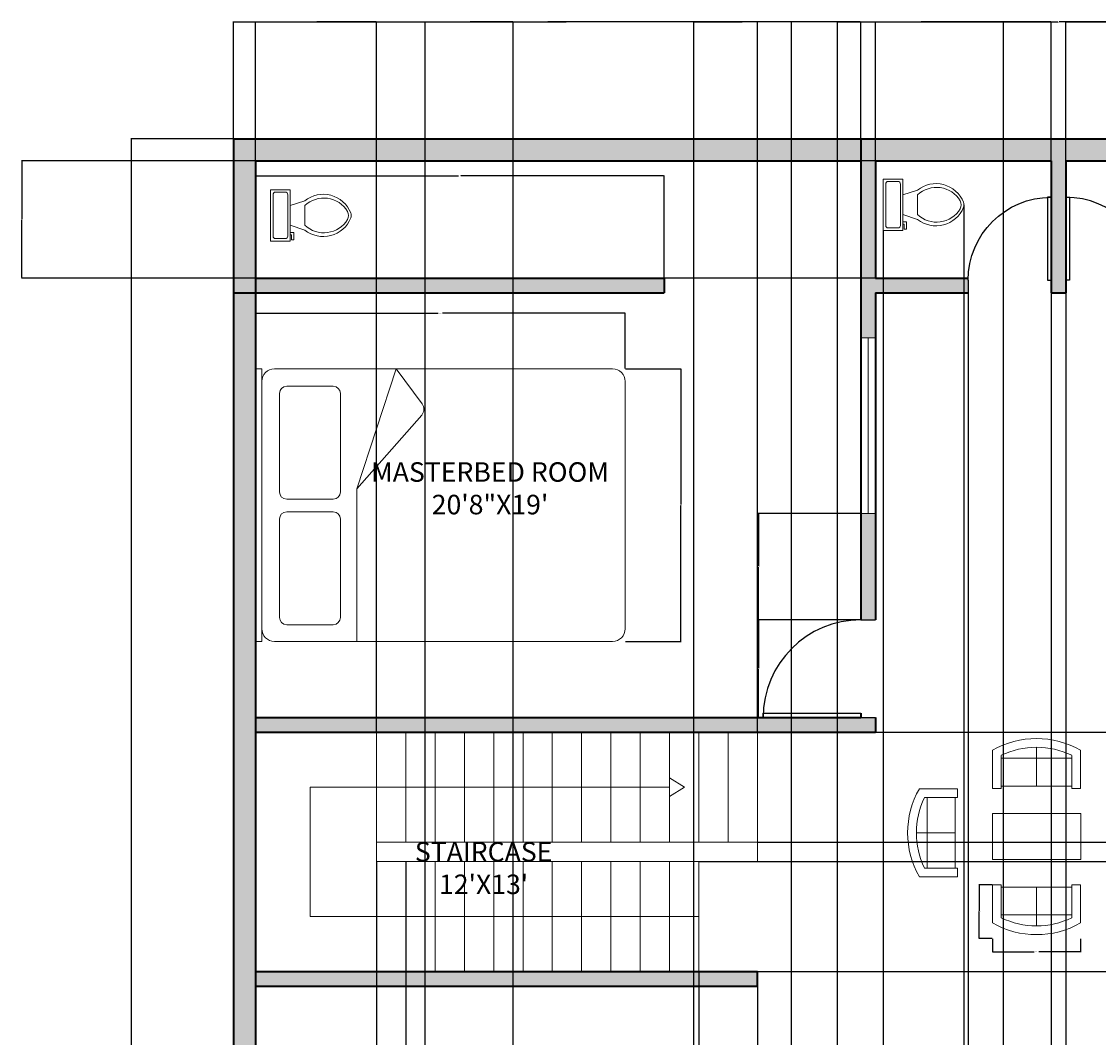
# Model space of a CAD drawing. Units: inches. Extents: x -89 to 661, y -827 to 77.
# Tile 4 of 5: x -89 to 353, y -339 to 77. Entities that reach past the tile are written whole.
import ezdxf

# ---------------------------------------------------------------- set-up
doc = ezdxf.new("R2010")
doc.units = ezdxf.units.IN
doc.header["$MEASUREMENT"] = 0
for name, color, linetype, lineweight in [('A-ANNO-DIMS', 2, 'Continuous', 18), ('A-AREA-IDEN', 7, 'Continuous', 18), ('A-FLOR-FIXT', 9, 'Continuous', 18), ('A-FLOR-STRS', 6, 'Continuous', 18), ('A-FURN', 34, 'Continuous', 18), ('A-GLAZ', 5, 'Continuous', 18), ('A-WALL', 7, 'Continuous', 35), ('A-WALL-PATT', 30, 'Continuous', 13), ('DOOR', 5, 'Continuous', 25)]:
    doc.layers.add(name, color=color, linetype=linetype, lineweight=lineweight)
doc.styles.get("Standard").update_dxf_attribs({"font": 'arial.ttf'})
doc.dimstyles.get("Standard").update_dxf_attribs({"dimtxt": 0.18, "dimasz": 0.18, "dimexe": 0.18, "dimexo": 0.0625, "dimgap": 0.09, "dimtad": 0, "dimtih": 1, "dimtoh": 1, "dimdec": 4, "dimzin": 0, "dimdsep": 46, "dimtxsty": 'Standard', "dimcen": 0.09, "dimadec": 0, "dimazin": 0, "dimtfac": 1, "dimtdec": 4, "dimtofl": 0, "dimtmove": 0, "dimatfit": 3, "dimfxl": 1, "dimtolj": 1, "dimtzin": 0, "dimarcsym": 0})

# ---------------------------------------------------------------- blocks, each defined once
blk = doc.blocks.new('*U7')
for p, q in [((0, 0), (0, -6)), ((40, 0), (40, -6))]:
    blk.add_line(p, q)
blk.add_lwpolyline([(0, 0), (0, 40), (1.75, 40), (1.75, 0)], close=True)
blk.add_arc((0, 0), 40, 0, 90)
blk = doc.blocks.new('A$C164346CA')
for p, q in [((0, 2.035), (0, 2)), ((1.5, 2.035), (0, 2.035)), ((1.5, 2), (1.5, 2.035)), ((1.5, 2), (0, 2)), ((0, 1.93), (0, 0.07)), ((0.6731, 1.9024), (0.1319, 1.9024)), ((1.364, 1.9024), (0.8228, 1.9024)), ((1.5, 0.07), (1.5, 1.93)), ((0.0919, 1.8624), (0.0919, 1.6069)), ((0.7131, 1.6069), (0.7131, 1.8624)), ((0.7828, 1.8624), (0.7828, 1.6069)), ((1.404, 1.6069), (1.404, 1.8624)), ((0.1319, 1.5669), (0.6731, 1.5669)), ((0.8228, 1.5669), (1.364, 1.5669)), ((0.8395, 1.4761), (0, 1.4761)), ((0.8395, 1.4761), (1.2448, 1.12)), ((1.5, 1.2611), (0.8395, 1.4761)), ((1.3077, 1.1175), (1.5, 1.2611)), ((0.07, 0), (1.43, 0))]:
    blk.add_line(p, q)
for centre, radius, start, end in [((0.07, 1.93), 0.07, 90, 180), ((1.43, 1.93), 0.07, 0, 90), ((0.1319, 1.8624), 0.04, 90, 180), ((0.6731, 1.8624), 0.04, 0, 90), ((0.8228, 1.8624), 0.04, 90, 180), ((1.364, 1.8624), 0.04, 0, 90), ((0.1319, 1.6069), 0.04, 180, 270), ((0.6731, 1.6069), 0.04, 270, 0), ((0.8228, 1.6069), 0.04, 180, 270), ((1.364, 1.6069), 0.04, 270, 0), ((1.2778, 1.1575), 0.05, 228.69584, 306.75789), ((0.07, 0.07), 0.07, 180, 270), ((1.43, 0.07), 0.07, 270, 0)]:
    blk.add_arc(centre, radius, start, end)
blk = doc.blocks.new('A$C01575E38')
for p, q in [((0, 0), (0, 0.65)), ((0, 0), (0, 0.65)), ((0.15, 0), (0.15, 0.563)), ((0.15, 0), (0.15, 0.563)), ((0.75, 0.039), (0.75, 0.7)), ((0.75, 0.039), (0.75, 0.7)), ((1.35, 0), (1.35, 0.563)), ((1.35, 0), (1.35, 0.563)), ((1.5, 0.65), (1.5, 0)), ((1.5, 0.65), (1.5, 0)), ((0.15, 0.515), (1.35, 0.515)), ((0.15, 0.515), (1.35, 0.515)), ((0.15, 0), (0, 0)), ((0.15, 0), (0, 0)), ((0.15, 0.039), (1.35, 0.039)), ((0.15, 0.039), (1.35, 0.039)), ((1.5, 0), (1.35, 0)), ((1.5, 0), (1.35, 0))]:
    blk.add_line(p, q)
for centre, radius, start, end in [((0.75, -0.656), 1.506, 60.1372, 119.8628), ((0.75, -0.656), 1.506, 60.1372, 119.8628), ((0.75, -0.685), 1.385, 64.3208, 115.6792), ((0.75, -0.685), 1.385, 64.3208, 115.6792)]:
    blk.add_arc(centre, radius, start, end)
blk = doc.blocks.new('*U15')
for p, q in [((9.5, -6), (9.5, -2)), ((-10, -8.5), (-8, -8.5)), ((-10, -9.5), (-10, -8.5)), ((-8, -8.5), (-8, -8)), ((-7, -8), (-7, -9.5)), ((-4, -8), (-6, -14)), ((4, -8), (6, -14)), ((-7, -9.5), (-10, -9.5)), ((4, -14), (-4, -14))]:
    blk.add_line(p, q)
blk.add_lwpolyline([(10.5, -8), (10.5, 0), (-10.5, 0), (-10.5, -8)], close=True)
for points in [[(-9.5, -2), (-9.5, -6)], [(8.5, -1), (-8.5, -1)], [(-8.5, -7), (8.5, -7)]]:
    blk.add_lwpolyline(points)
for centre, radius, start, end in [((-8.62, -1.88), 0.884, 81.8699, 188.1301), ((8.62, -1.88), 0.884, 351.8699, 98.1301), ((-8.62, -6.12), 0.884, 171.8699, 278.1301), ((8.62, -6.12), 0.884, 261.8699, 8.1301), ((3.52, -21.58), 12.17, 141.4691, 247.9714), ((4.2, -21.82), 11.33, 136.3677, 238.9468), ((-3.52, -21.58), 12.17, 292.0284, 38.5307), ((-4.2, -21.82), 11.33, 301.053, 43.6321), ((0, -27.88), 4, 245.7318, 294.2682), ((0, -29), 4, 254.8605, 285.1395)]:
    blk.add_arc(centre, radius, start, end)
blk = doc.blocks.new('WIN-72-NOM')
for p, q in [((0, 6), (0, 0)), ((0, 6), (71.86, 6)), ((71.86, 6), (71.86, 0)), ((0, 3), (71.86, 3)), ((0, 0), (71.86, 0))]:
    blk.add_line(p, q)
blk = doc.blocks.new('*D17')
at = {"layer": 'A-ANNO-DIMS', "color": 0, "lineweight": -2, "transparency": 16777216}
for p, q in [((309.15, -298.56), (309.15, -304.09)), ((345.23, -298.56), (345.23, -304.09)), ((309.33, -303.91), (326.24, -303.91)), ((345.05, -303.91), (328.14, -303.91))]:
    blk.add_line(p, q, dxfattribs=at)
at = {"layer": 'A-ANNO-DIMS', "color": 0, "transparency": 16777216}
for points in [[(309.33, -303.88), (309.33, -303.94), (309.15, -303.91)], [(345.05, -303.88), (345.05, -303.94), (345.23, -303.91)]]:
    blk.add_solid(points, dxfattribs=at)
at = {"layer": 'Defpoints', "color": 0, "transparency": 16777216}
for p in [(309.15, -298.49), (345.23, -298.49), (345.23, -303.91)]:
    blk.add_point(p, dxfattribs=at)
at = {"layer": 'A-ANNO-DIMS', "color": 0, "transparency": 16777216, "insert": (327.19, -303.91), "char_height": 0.18, "attachment_point": 5}
blk.add_mtext('\\A1;CHAIR 36 TYP.', dxfattribs=at)
blk = doc.blocks.new('*D18')
at = {"layer": 'A-ANNO-DIMS', "color": 0, "lineweight": -2, "transparency": 16777216}
for p, q in [((309.09, -276.45), (303.56, -276.45)), ((303.74, -276.63), (303.74, -287.29)), ((303.74, -298.31), (303.74, -287.65)), ((309.09, -298.49), (303.56, -298.49))]:
    blk.add_line(p, q, dxfattribs=at)
at = {"layer": 'A-ANNO-DIMS', "color": 0, "transparency": 16777216}
for points in [[(303.71, -276.63), (303.77, -276.63), (303.74, -276.45)], [(303.71, -298.31), (303.77, -298.31), (303.74, -298.49)]]:
    blk.add_solid(points, dxfattribs=at)
at = {"layer": 'Defpoints', "color": 0, "transparency": 16777216}
for p in [(309.15, -276.45), (303.74, -298.49), (309.15, -298.49)]:
    blk.add_point(p, dxfattribs=at)
at = {"layer": 'A-ANNO-DIMS', "color": 0, "transparency": 16777216, "insert": (303.74, -287.47), "char_height": 0.18, "attachment_point": 5}
blk.add_mtext('\\A1;22 TYP.', dxfattribs=at)
blk = doc.blocks.new('*D21')
at = {"layer": 'A-ANNO-DIMS', "color": 0, "lineweight": -2, "transparency": 16777216}
for p, q in [((7.19, -65.04), (7.19, -42.19)), ((7.37, -42.37), (82.06, -42.37)), ((158.52, -42.37), (83.83, -42.37)), ((158.7, -65.04), (158.7, -42.19))]:
    blk.add_line(p, q, dxfattribs=at)
at = {"layer": 'A-ANNO-DIMS', "color": 0, "transparency": 16777216}
for points in [[(7.37, -42.34), (7.37, -42.4), (7.19, -42.37)], [(158.52, -42.34), (158.52, -42.4), (158.7, -42.37)]]:
    blk.add_solid(points, dxfattribs=at)
at = {"layer": 'Defpoints', "color": 0, "transparency": 16777216}
for p in [(7.19, -42.37), (7.19, -65.1), (158.7, -65.1)]:
    blk.add_point(p, dxfattribs=at)
at = {"layer": 'A-ANNO-DIMS', "color": 0, "transparency": 16777216, "insert": (82.94, -42.37), "char_height": 0.18, "attachment_point": 5}
blk.add_mtext('\\A1;BED 152 TYP.', dxfattribs=at)
blk = doc.blocks.new('*D22')
at = {"layer": 'A-ANNO-DIMS', "color": 0, "lineweight": -2, "transparency": 16777216}
for p, q in [((158.76, -65.1), (181.61, -65.1)), ((181.43, -65.28), (181.43, -120.76)), ((181.43, -176.6), (181.43, -121.12)), ((158.76, -176.78), (181.61, -176.78))]:
    blk.add_line(p, q, dxfattribs=at)
at = {"layer": 'A-ANNO-DIMS', "color": 0, "transparency": 16777216}
for points in [[(181.4, -65.28), (181.46, -65.28), (181.43, -65.1)], [(181.4, -176.6), (181.46, -176.6), (181.43, -176.78)]]:
    blk.add_solid(points, dxfattribs=at)
at = {"layer": 'Defpoints', "color": 0, "transparency": 16777216}
for p in [(158.7, -65.1), (181.43, -65.1), (158.7, -176.78)]:
    blk.add_point(p, dxfattribs=at)
at = {"layer": 'A-ANNO-DIMS', "color": 0, "transparency": 16777216, "insert": (181.43, -120.94), "char_height": 0.18, "attachment_point": 5}
blk.add_mtext('\\A1;112 TYP.', dxfattribs=at)
blk = doc.blocks.new('*D32')
at = {"layer": 'A-ANNO-DIMS', "color": 0, "lineweight": -2, "transparency": 16777216}
for p, q in [((-1.88, 29.06), (-43.85, 29.06)), ((-43.67, 28.88), (-43.67, -376.76)), ((-43.67, -782.76), (-43.67, -377.12)), ((-1.88, -782.94), (-43.85, -782.94))]:
    blk.add_line(p, q, dxfattribs=at)
at = {"layer": 'A-ANNO-DIMS', "color": 0, "transparency": 16777216}
for points in [[(-43.7, 28.88), (-43.64, 28.88), (-43.67, 29.06)], [(-43.7, -782.76), (-43.64, -782.76), (-43.67, -782.94)]]:
    blk.add_solid(points, dxfattribs=at)
at = {"layer": 'Defpoints', "color": 0, "transparency": 16777216}
for p in [(-43.67, 29.06), (-1.81, 29.06), (-1.81, -782.94)]:
    blk.add_point(p, dxfattribs=at)
at = {"layer": 'A-ANNO-DIMS', "color": 0, "transparency": 16777216, "insert": (-43.67, -376.94), "char_height": 0.18, "attachment_point": 5}
blk.add_mtext('\\A1;812', dxfattribs=at)
blk = doc.blocks.new('*D33')
at = {"layer": 'A-ANNO-DIMS', "color": 0, "lineweight": -2, "transparency": 16777216}
for p, q in [((-1.81, 29.12), (-1.81, 77.13)), ((-1.63, 76.95), (126.4, 76.95)), ((255.01, 76.95), (126.98, 76.95)), ((255.19, 29.12), (255.19, 77.13))]:
    blk.add_line(p, q, dxfattribs=at)
at = {"layer": 'A-ANNO-DIMS', "color": 0, "transparency": 16777216}
for points in [[(-1.63, 76.98), (-1.63, 76.92), (-1.81, 76.95)], [(255.01, 76.98), (255.01, 76.92), (255.19, 76.95)]]:
    blk.add_solid(points, dxfattribs=at)
at = {"layer": 'Defpoints', "color": 0, "transparency": 16777216}
for p in [(255.19, 76.95), (-1.81, 29.06), (255.19, 29.06)]:
    blk.add_point(p, dxfattribs=at)
at = {"layer": 'A-ANNO-DIMS', "color": 0, "transparency": 16777216, "insert": (126.69, 76.95), "char_height": 0.18, "attachment_point": 5}
blk.add_mtext('\\A1;257', dxfattribs=at)
blk = doc.blocks.new('*D41')
at = {"layer": 'A-ANNO-DIMS', "color": 0, "lineweight": -2, "transparency": 16777216}
for p, q in [((255.19, 29.12), (255.19, 77.13)), ((255.37, 76.95), (335.91, 76.95)), ((417.01, 76.95), (336.47, 76.95)), ((417.19, 29.12), (417.19, 77.13))]:
    blk.add_line(p, q, dxfattribs=at)
at = {"layer": 'A-ANNO-DIMS', "color": 0, "transparency": 16777216}
for points in [[(255.37, 76.98), (255.37, 76.92), (255.19, 76.95)], [(417.01, 76.98), (417.01, 76.92), (417.19, 76.95)]]:
    blk.add_solid(points, dxfattribs=at)
at = {"layer": 'Defpoints', "color": 0, "transparency": 16777216}
for p in [(417.19, 76.95), (255.19, 29.06), (417.19, 29.06)]:
    blk.add_point(p, dxfattribs=at)
at = {"layer": 'A-ANNO-DIMS', "color": 0, "transparency": 16777216, "insert": (336.19, 76.95), "char_height": 0.18, "attachment_point": 5}
blk.add_mtext('\\A1;162', dxfattribs=at)
blk = doc.blocks.new('*D42')
at = {"layer": 'A-ANNO-DIMS', "color": 0, "lineweight": -2, "transparency": 16777216}
for p, q in [((261.19, 20.12), (261.19, 77.13)), ((261.37, 76.95), (296.97, 76.95)), ((333.01, 76.95), (297.4, 76.95)), ((333.19, 20.12), (333.19, 77.13))]:
    blk.add_line(p, q, dxfattribs=at)
at = {"layer": 'A-ANNO-DIMS', "color": 0, "transparency": 16777216}
for points in [[(261.37, 76.98), (261.37, 76.92), (261.19, 76.95)], [(333.01, 76.98), (333.01, 76.92), (333.19, 76.95)]]:
    blk.add_solid(points, dxfattribs=at)
at = {"layer": 'Defpoints', "color": 0, "transparency": 16777216}
for p in [(333.19, 76.95), (261.19, 20.06), (333.19, 20.06)]:
    blk.add_point(p, dxfattribs=at)
at = {"layer": 'A-ANNO-DIMS', "color": 0, "transparency": 16777216, "insert": (297.19, 76.95), "char_height": 0.18, "attachment_point": 5}
blk.add_mtext('\\A1;72', dxfattribs=at)
blk = doc.blocks.new('*D43')
at = {"layer": 'A-ANNO-DIMS', "color": 0, "lineweight": -2, "transparency": 16777216}
for p, q in [((261.12, 20.06), (-88.61, 20.06)), ((-88.43, 19.88), (-88.43, -3.76)), ((-88.43, -27.76), (-88.43, -4.12)), ((261.12, -27.94), (-88.61, -27.94))]:
    blk.add_line(p, q, dxfattribs=at)
at = {"layer": 'A-ANNO-DIMS', "color": 0, "transparency": 16777216}
for points in [[(-88.46, 19.88), (-88.4, 19.88), (-88.43, 20.06)], [(-88.46, -27.76), (-88.4, -27.76), (-88.43, -27.94)]]:
    blk.add_solid(points, dxfattribs=at)
at = {"layer": 'Defpoints', "color": 0, "transparency": 16777216}
for p in [(-88.43, 20.06), (261.19, 20.06), (261.19, -27.94)]:
    blk.add_point(p, dxfattribs=at)
at = {"layer": 'A-ANNO-DIMS', "color": 0, "transparency": 16777216, "insert": (-88.43, -3.94), "char_height": 0.18, "attachment_point": 5}
blk.add_mtext('\\A1;48', dxfattribs=at)
blk = doc.blocks.new('*D44')
at = {"layer": 'A-ANNO-DIMS', "color": 0, "lineweight": -2, "transparency": 16777216}
for p, q in [((299.19, -34), (299.19, -826.85)), ((333.19, -34), (333.19, -826.85)), ((299.37, -826.67), (315.97, -826.67)), ((333.01, -826.67), (316.4, -826.67))]:
    blk.add_line(p, q, dxfattribs=at)
at = {"layer": 'A-ANNO-DIMS', "color": 0, "transparency": 16777216}
for points in [[(299.37, -826.64), (299.37, -826.7), (299.19, -826.67)], [(333.01, -826.64), (333.01, -826.7), (333.19, -826.67)]]:
    blk.add_solid(points, dxfattribs=at)
at = {"layer": 'Defpoints', "color": 0, "transparency": 16777216}
for p in [(299.19, -33.94), (333.19, -33.94), (333.19, -826.67)]:
    blk.add_point(p, dxfattribs=at)
at = {"layer": 'A-ANNO-DIMS', "color": 0, "transparency": 16777216, "insert": (316.19, -826.67), "char_height": 0.18, "attachment_point": 5}
blk.add_mtext('\\A1;34', dxfattribs=at)
blk = doc.blocks.new('*D45')
at = {"layer": 'A-ANNO-DIMS', "color": 0, "lineweight": -2, "transparency": 16777216}
for p, q in [((339.19, 20.12), (339.19, 77.13)), ((339.37, 76.95), (374.97, 76.95)), ((411.01, 76.95), (375.4, 76.95)), ((411.19, 20.12), (411.19, 77.13))]:
    blk.add_line(p, q, dxfattribs=at)
at = {"layer": 'A-ANNO-DIMS', "color": 0, "transparency": 16777216}
for points in [[(339.37, 76.98), (339.37, 76.92), (339.19, 76.95)], [(411.01, 76.98), (411.01, 76.92), (411.19, 76.95)]]:
    blk.add_solid(points, dxfattribs=at)
at = {"layer": 'Defpoints', "color": 0, "transparency": 16777216}
for p in [(411.19, 76.95), (339.19, 20.06), (411.19, 20.06)]:
    blk.add_point(p, dxfattribs=at)
at = {"layer": 'A-ANNO-DIMS', "color": 0, "transparency": 16777216, "insert": (375.19, 76.95), "char_height": 0.18, "attachment_point": 5}
blk.add_mtext('\\A1;72', dxfattribs=at)
blk = doc.blocks.new('*D46')
at = {"layer": 'A-ANNO-DIMS', "color": 0, "lineweight": -2, "transparency": 16777216}
for p, q in [((333.19, -34), (333.19, -826.85)), ((339.19, -34), (339.19, -826.85)), ((333.37, -826.67), (336.04, -826.67)), ((339.01, -826.67), (336.34, -826.67))]:
    blk.add_line(p, q, dxfattribs=at)
at = {"layer": 'A-ANNO-DIMS', "color": 0, "transparency": 16777216}
for points in [[(333.37, -826.64), (333.37, -826.7), (333.19, -826.67)], [(339.01, -826.64), (339.01, -826.7), (339.19, -826.67)]]:
    blk.add_solid(points, dxfattribs=at)
at = {"layer": 'Defpoints', "color": 0, "transparency": 16777216}
for p in [(333.19, -33.94), (339.19, -33.94), (339.19, -826.67)]:
    blk.add_point(p, dxfattribs=at)
at = {"layer": 'A-ANNO-DIMS', "color": 0, "transparency": 16777216, "insert": (336.19, -826.67), "char_height": 0.18, "attachment_point": 5}
blk.add_mtext('\\A1;6', dxfattribs=at)
blk = doc.blocks.new('*D48')
at = {"layer": 'A-ANNO-DIMS', "color": 0, "lineweight": -2, "transparency": 16777216}
for p, q in [((297.44, 2.03), (297.44, -826.85)), ((264.44, -8.47), (264.44, -826.85)), ((264.62, -826.67), (280.72, -826.67)), ((297.26, -826.67), (281.15, -826.67))]:
    blk.add_line(p, q, dxfattribs=at)
at = {"layer": 'A-ANNO-DIMS', "color": 0, "transparency": 16777216}
for points in [[(264.62, -826.64), (264.62, -826.7), (264.44, -826.67)], [(297.26, -826.64), (297.26, -826.7), (297.44, -826.67)]]:
    blk.add_solid(points, dxfattribs=at)
at = {"layer": 'Defpoints', "color": 0, "transparency": 16777216}
for p in [(297.44, 2.09), (264.44, -8.41), (297.44, -826.67)]:
    blk.add_point(p, dxfattribs=at)
at = {"layer": 'A-ANNO-DIMS', "color": 0, "transparency": 16777216, "insert": (280.94, -826.67), "char_height": 0.18, "attachment_point": 5}
blk.add_mtext('\\A1;33', dxfattribs=at)
blk = doc.blocks.new('*D50')
at = {"layer": 'A-ANNO-DIMS', "color": 0, "lineweight": -2, "transparency": 16777216}
for p, q in [((212.9, -213.94), (661.23, -213.94)), ((661.05, -214.12), (661.05, -236.26)), ((661.05, -258.76), (661.05, -236.62)), ((212.9, -258.94), (661.23, -258.94))]:
    blk.add_line(p, q, dxfattribs=at)
at = {"layer": 'A-ANNO-DIMS', "color": 0, "transparency": 16777216}
for points in [[(661.02, -214.12), (661.08, -214.12), (661.05, -213.94)], [(661.02, -258.76), (661.08, -258.76), (661.05, -258.94)]]:
    blk.add_solid(points, dxfattribs=at)
at = {"layer": 'Defpoints', "color": 0, "transparency": 16777216}
for p in [(212.84, -213.94), (661.05, -213.94), (212.84, -258.94)]:
    blk.add_point(p, dxfattribs=at)
at = {"layer": 'A-ANNO-DIMS', "color": 0, "transparency": 16777216, "insert": (661.05, -236.44), "char_height": 0.18, "attachment_point": 5}
blk.add_mtext('\\A1;45', dxfattribs=at)
blk = doc.blocks.new('*D51')
at = {"layer": 'A-ANNO-DIMS', "color": 0, "lineweight": -2, "transparency": 16777216}
for p, q in [((188.9, -266.94), (661.23, -266.94)), ((661.05, -267.12), (661.05, -289.26)), ((661.05, -311.76), (661.05, -289.62)), ((188.9, -311.94), (661.23, -311.94))]:
    blk.add_line(p, q, dxfattribs=at)
at = {"layer": 'A-ANNO-DIMS', "color": 0, "transparency": 16777216}
for points in [[(661.02, -267.12), (661.08, -267.12), (661.05, -266.94)], [(661.02, -311.76), (661.08, -311.76), (661.05, -311.94)]]:
    blk.add_solid(points, dxfattribs=at)
at = {"layer": 'Defpoints', "color": 0, "transparency": 16777216}
for p in [(188.84, -266.94), (661.05, -266.94), (188.84, -311.94)]:
    blk.add_point(p, dxfattribs=at)
at = {"layer": 'A-ANNO-DIMS', "color": 0, "transparency": 16777216, "insert": (661.05, -289.44), "char_height": 0.18, "attachment_point": 5}
blk.add_mtext('\\A1;45', dxfattribs=at)
blk = doc.blocks.new('*D52')
at = {"layer": 'A-ANNO-DIMS', "color": 0, "lineweight": -2, "transparency": 16777216}
for p, q in [((212.9, -258.94), (661.23, -258.94)), ((661.05, -259.12), (661.05, -262.76)), ((661.05, -266.76), (661.05, -263.12)), ((212.9, -266.94), (661.23, -266.94))]:
    blk.add_line(p, q, dxfattribs=at)
at = {"layer": 'A-ANNO-DIMS', "color": 0, "transparency": 16777216}
for points in [[(661.02, -259.12), (661.08, -259.12), (661.05, -258.94)], [(661.02, -266.76), (661.08, -266.76), (661.05, -266.94)]]:
    blk.add_solid(points, dxfattribs=at)
at = {"layer": 'Defpoints', "color": 0, "transparency": 16777216}
for p in [(212.84, -258.94), (661.05, -258.94), (212.84, -266.94)]:
    blk.add_point(p, dxfattribs=at)
at = {"layer": 'A-ANNO-DIMS', "color": 0, "transparency": 16777216, "insert": (661.05, -262.94), "char_height": 0.18, "attachment_point": 5}
blk.add_mtext('\\A1;8', dxfattribs=at)
blk = doc.blocks.new('*D53')
at = {"layer": 'A-ANNO-DIMS', "color": 0, "lineweight": -2, "transparency": 16777216}
for p, q in [((7.19, -213.88), (7.19, 77.13)), ((7.37, 76.95), (31.61, 76.95)), ((56.66, 76.95), (32.41, 76.95)), ((56.84, -213.88), (56.84, 77.13))]:
    blk.add_line(p, q, dxfattribs=at)
at = {"layer": 'A-ANNO-DIMS', "color": 0, "transparency": 16777216}
for points in [[(7.37, 76.98), (7.37, 76.92), (7.19, 76.95)], [(56.66, 76.98), (56.66, 76.92), (56.84, 76.95)]]:
    blk.add_solid(points, dxfattribs=at)
at = {"layer": 'Defpoints', "color": 0, "transparency": 16777216}
for p in [(56.84, 76.95), (7.19, -213.94), (56.84, -213.94)]:
    blk.add_point(p, dxfattribs=at)
at = {"layer": 'A-ANNO-DIMS', "color": 0, "transparency": 16777216, "insert": (32.01, 76.95), "char_height": 0.18, "attachment_point": 5}
blk.add_mtext('\\A1;49.65', dxfattribs=at)
blk = doc.blocks.new('*D54')
at = {"layer": 'A-ANNO-DIMS', "color": 0, "lineweight": -2, "transparency": 16777216}
for p, q in [((56.84, -213.88), (56.84, 77.13)), ((57.02, 76.95), (134.56, 76.95)), ((212.66, 76.95), (135.12, 76.95)), ((212.84, -213.88), (212.84, 77.13))]:
    blk.add_line(p, q, dxfattribs=at)
at = {"layer": 'A-ANNO-DIMS', "color": 0, "transparency": 16777216}
for points in [[(57.02, 76.98), (57.02, 76.92), (56.84, 76.95)], [(212.66, 76.98), (212.66, 76.92), (212.84, 76.95)]]:
    blk.add_solid(points, dxfattribs=at)
at = {"layer": 'Defpoints', "color": 0, "transparency": 16777216}
for p in [(212.84, 76.95), (56.84, -213.94), (212.84, -213.94)]:
    blk.add_point(p, dxfattribs=at)
at = {"layer": 'A-ANNO-DIMS', "color": 0, "transparency": 16777216, "insert": (134.84, 76.95), "char_height": 0.18, "attachment_point": 5}
blk.add_mtext('\\A1;156', dxfattribs=at)
blk = doc.blocks.new('*D55')
at = {"layer": 'A-ANNO-DIMS', "color": 0, "lineweight": -2, "transparency": 16777216}
for p, q in [((56.84, -267), (56.84, -826.85)), ((68.84, -267), (68.84, -826.85)), ((57.02, -826.67), (62.63, -826.67)), ((68.66, -826.67), (63.05, -826.67))]:
    blk.add_line(p, q, dxfattribs=at)
at = {"layer": 'A-ANNO-DIMS', "color": 0, "transparency": 16777216}
for points in [[(57.02, -826.64), (57.02, -826.7), (56.84, -826.67)], [(68.66, -826.64), (68.66, -826.7), (68.84, -826.67)]]:
    blk.add_solid(points, dxfattribs=at)
at = {"layer": 'Defpoints', "color": 0, "transparency": 16777216}
for p in [(56.84, -266.94), (68.84, -266.94), (68.84, -826.67)]:
    blk.add_point(p, dxfattribs=at)
at = {"layer": 'A-ANNO-DIMS', "color": 0, "transparency": 16777216, "insert": (62.84, -826.67), "char_height": 0.18, "attachment_point": 5}
blk.add_mtext('\\A1;12', dxfattribs=at)
blk = doc.blocks.new('*D56')
at = {"layer": 'A-ANNO-DIMS', "color": 0, "lineweight": -2, "transparency": 16777216}
for p, q in [((188.84, -312), (188.84, -826.85)), ((212.84, -318), (212.84, -826.85)), ((189.02, -826.67), (200.62, -826.67)), ((212.66, -826.67), (201.06, -826.67))]:
    blk.add_line(p, q, dxfattribs=at)
at = {"layer": 'A-ANNO-DIMS', "color": 0, "transparency": 16777216}
for points in [[(189.02, -826.64), (189.02, -826.7), (188.84, -826.67)], [(212.66, -826.64), (212.66, -826.7), (212.84, -826.67)]]:
    blk.add_solid(points, dxfattribs=at)
at = {"layer": 'Defpoints', "color": 0, "transparency": 16777216}
for p in [(188.84, -311.94), (212.84, -317.94), (212.84, -826.67)]:
    blk.add_point(p, dxfattribs=at)
at = {"layer": 'A-ANNO-DIMS', "color": 0, "transparency": 16777216, "insert": (200.84, -826.67), "char_height": 0.18, "attachment_point": 5}
blk.add_mtext('\\A1;24', dxfattribs=at)
blk = doc.blocks.new('*D61')
at = {"layer": 'A-ANNO-DIMS', "color": 0, "lineweight": -2, "transparency": 16777216}
for p, q in [((245.68, -494.78), (245.68, 77.13)), ((245.86, 76.95), (279.46, 76.95)), ((313.5, 76.95), (279.9, 76.95)), ((313.68, -494.78), (313.68, 77.13))]:
    blk.add_line(p, q, dxfattribs=at)
at = {"layer": 'A-ANNO-DIMS', "color": 0, "transparency": 16777216}
for points in [[(245.86, 76.98), (245.86, 76.92), (245.68, 76.95)], [(313.5, 76.98), (313.5, 76.92), (313.68, 76.95)]]:
    blk.add_solid(points, dxfattribs=at)
at = {"layer": 'Defpoints', "color": 0, "transparency": 16777216}
for p in [(313.68, 76.95), (245.68, -494.84), (313.68, -494.84)]:
    blk.add_point(p, dxfattribs=at)
at = {"layer": 'A-ANNO-DIMS', "color": 0, "transparency": 16777216, "insert": (279.68, 76.95), "char_height": 0.18, "attachment_point": 5}
blk.add_mtext('\\A1;68', dxfattribs=at)
blk = doc.blocks.new('*D62')
at = {"layer": 'A-ANNO-DIMS', "color": 0, "lineweight": -2, "transparency": 16777216}
for p, q in [((186.79, -527.88), (186.79, 77.13)), ((186.97, 76.95), (206.57, 76.95)), ((226.61, 76.95), (207.01, 76.95)), ((226.79, -527.88), (226.79, 77.13))]:
    blk.add_line(p, q, dxfattribs=at)
at = {"layer": 'A-ANNO-DIMS', "color": 0, "transparency": 16777216}
for points in [[(186.97, 76.98), (186.97, 76.92), (186.79, 76.95)], [(226.61, 76.98), (226.61, 76.92), (226.79, 76.95)]]:
    blk.add_solid(points, dxfattribs=at)
at = {"layer": 'Defpoints', "color": 0, "transparency": 16777216}
for p in [(226.79, 76.95), (186.79, -527.94), (226.79, -527.94)]:
    blk.add_point(p, dxfattribs=at)
at = {"layer": 'A-ANNO-DIMS', "color": 0, "transparency": 16777216, "insert": (206.79, 76.95), "char_height": 0.18, "attachment_point": 5}
blk.add_mtext('\\A1;40', dxfattribs=at)
blk = doc.blocks.new('*D64')
at = {"layer": 'A-ANNO-DIMS', "color": 0, "lineweight": -2, "transparency": 16777216}
for p, q in [((255.12, -167.94), (213.15, -167.94)), ((213.33, -168.12), (213.33, -187.76)), ((213.33, -207.76), (213.33, -188.12)), ((255.12, -207.94), (213.15, -207.94))]:
    blk.add_line(p, q, dxfattribs=at)
at = {"layer": 'A-ANNO-DIMS', "color": 0, "transparency": 16777216}
for points in [[(213.3, -168.12), (213.36, -168.12), (213.33, -167.94)], [(213.3, -207.76), (213.36, -207.76), (213.33, -207.94)]]:
    blk.add_solid(points, dxfattribs=at)
at = {"layer": 'Defpoints', "color": 0, "transparency": 16777216}
for p in [(213.33, -167.94), (255.19, -167.94), (255.19, -207.94)]:
    blk.add_point(p, dxfattribs=at)
at = {"layer": 'A-ANNO-DIMS', "color": 0, "transparency": 16777216, "insert": (213.33, -187.94), "char_height": 0.18, "attachment_point": 5}
blk.add_mtext('\\A1;40', dxfattribs=at)
blk = doc.blocks.new('*D69')
at = {"layer": 'A-ANNO-DIMS', "color": 0, "lineweight": -2, "transparency": 16777216}
for p, q in [((76.79, -629.88), (76.79, 77.13)), ((76.97, 76.95), (94.39, 76.95)), ((112.59, 76.95), (95.17, 76.95)), ((112.77, -629.88), (112.77, 77.13))]:
    blk.add_line(p, q, dxfattribs=at)
at = {"layer": 'A-ANNO-DIMS', "color": 0, "transparency": 16777216}
for points in [[(76.97, 76.98), (76.97, 76.92), (76.79, 76.95)], [(112.59, 76.98), (112.59, 76.92), (112.77, 76.95)]]:
    blk.add_solid(points, dxfattribs=at)
at = {"layer": 'Defpoints', "color": 0, "transparency": 16777216}
for p in [(112.77, 76.95), (76.79, -629.94), (112.77, -629.94)]:
    blk.add_point(p, dxfattribs=at)
at = {"layer": 'A-ANNO-DIMS', "color": 0, "transparency": 16777216, "insert": (94.78, 76.95), "char_height": 0.18, "attachment_point": 5}
blk.add_mtext('\\A1;35.98', dxfattribs=at)
blk = doc.blocks.new('*D70')
at = {"layer": 'A-ANNO-DIMS', "color": 0, "lineweight": -2, "transparency": 16777216}
for p, q in [((255.12, -124.33), (213.15, -124.33)), ((213.33, -124.51), (213.33, -145.95)), ((213.33, -167.76), (213.33, -146.32)), ((255.12, -167.94), (213.15, -167.94))]:
    blk.add_line(p, q, dxfattribs=at)
at = {"layer": 'A-ANNO-DIMS', "color": 0, "transparency": 16777216}
for points in [[(213.3, -124.51), (213.36, -124.51), (213.33, -124.33)], [(213.3, -167.76), (213.36, -167.76), (213.33, -167.94)]]:
    blk.add_solid(points, dxfattribs=at)
at = {"layer": 'Defpoints', "color": 0, "transparency": 16777216}
for p in [(213.33, -124.33), (255.19, -124.33), (255.19, -167.94)]:
    blk.add_point(p, dxfattribs=at)
at = {"layer": 'A-ANNO-DIMS', "color": 0, "transparency": 16777216, "insert": (213.33, -146.13), "char_height": 0.18, "attachment_point": 5}
blk.add_mtext('\\A1;43.61', dxfattribs=at)
blk = doc.blocks.new('*D75')
at = {"layer": 'A-ANNO-DIMS', "color": 0, "lineweight": -2, "transparency": 16777216}
for p, q in [((7.19, -27.88), (7.19, 14.1)), ((7.37, 13.92), (90.45, 13.92)), ((174.44, 13.92), (91.36, 13.92)), ((174.62, -27.88), (174.62, 14.1))]:
    blk.add_line(p, q, dxfattribs=at)
at = {"layer": 'A-ANNO-DIMS', "color": 0, "transparency": 16777216}
for points in [[(7.37, 13.95), (7.37, 13.89), (7.19, 13.92)], [(174.44, 13.95), (174.44, 13.89), (174.62, 13.92)]]:
    blk.add_solid(points, dxfattribs=at)
at = {"layer": 'Defpoints', "color": 0, "transparency": 16777216}
for p in [(174.62, 13.92), (7.19, -27.94), (174.62, -27.94)]:
    blk.add_point(p, dxfattribs=at)
at = {"layer": 'A-ANNO-DIMS', "color": 0, "transparency": 16777216, "insert": (90.9, 13.92), "char_height": 0.18, "attachment_point": 5}
blk.add_mtext('\\A1;167.43', dxfattribs=at)

msp = doc.modelspace()

# ---------------------------------------------------------------- hatches: boundary and pattern name
at = {"layer": 'A-WALL-PATT'}
h = msp.add_hatch(color=256, dxfattribs=at)
h.dxf.hatch_style = 1
h.paths.add_polyline_path([(255.186, 29.06), (-1.814, 29.06), (-1.814, -33.94), (7.186, -33.94), (7.186, -27.94), (7.186, 20.06), (255.186, 20.06)])
h.paths.add_polyline_path([(174.616, -27.94), (7.186, -27.94), (7.186, -33.94), (174.616, -33.94)], flags=17)
h.paths.add_polyline_path([(7.186, -33.94), (-1.814, -33.94), (-1.814, -527.94), (7.186, -527.94), (7.186, -425.94), (7.186, -311.94), (7.186, -207.94)])
h.paths.add_polyline_path([(7.186, -527.94), (-1.814, -527.94), (-1.814, -782.94), (430.186, -782.94), (430.186, -773.94), (7.186, -773.94)])
h = msp.add_hatch(color=256, dxfattribs=at)
h.dxf.hatch_style = 1
h.paths.add_polyline_path([(610.186, -311.94), (417.186, -311.94), (417.186, -288.111), (411.186, -288.111), (411.186, -317.94), (610.186, -317.94)])
h.paths.add_polyline_path([(417.186, -188.94), (411.186, -188.94), (411.186, -216.247), (417.186, -216.247)])
h.paths.add_polyline_path([(610.186, -142.94), (417.186, -142.94), (411.186, -142.94), (411.186, -148.94), (417.186, -148.94), (457.186, -148.94), (610.186, -148.94)])
h.paths.add_polyline_path([(417.186, -82.701), (411.186, -82.701), (411.186, -102.94), (417.186, -102.94)])
h.paths.add_polyline_path([(261.186, -124.327), (255.186, -124.327), (255.186, -167.94), (261.186, -167.94)])
h.paths.add_polyline_path([(261.186, 20.06), (333.186, 20.06), (333.186, -33.94), (339.186, -33.94), (339.186, -28.84), (339.186, 5.16), (339.186, 20.06), (411.186, 20.06), (411.186, -27.94), (373.174, -27.94, -0.0066185), (373.186, -28.84), (373.186, -33.94), (411.186, -33.94), (411.186, -46.769), (417.186, -46.769), (417.186, 29.06), (255.186, 29.06), (255.186, -52.464), (261.186, -52.464), (261.186, -33.94), (299.186, -33.94), (299.186, -28.84, -0.0066185), (299.198, -27.94), (261.186, -27.94)])
h.paths.add_polyline_path([(261.186, -207.94), (255.186, -207.94), (215.186, -207.94), (7.186, -207.94), (7.186, -213.94), (261.186, -213.94)])
h.paths.add_polyline_path([(212.837, -311.94), (7.186, -311.94), (7.186, -317.94), (212.837, -317.94)])

# ---------------------------------------------------------------- linework, layer by layer
at = {"layer": 'A-FLOR-STRS'}
for p, q in [((56.837, -311.94), (56.837, -213.94)), ((68.837, -258.94), (68.837, -213.94)), ((80.837, -258.94), (80.837, -213.94)), ((92.837, -258.94), (92.837, -213.94)), ((104.837, -258.94), (104.837, -213.94)), ((116.837, -258.94), (116.837, -213.94)), ((128.837, -258.94), (128.837, -213.94)), ((140.837, -258.94), (140.837, -213.94)), ((152.837, -258.94), (152.837, -213.94)), ((164.837, -258.94), (164.837, -213.94)), ((176.837, -258.94), (176.837, -213.94)), ((188.837, -258.94), (188.837, -213.94)), ((200.837, -258.94), (200.837, -213.94)), ((212.837, -266.94), (212.837, -213.94)), ((176.837, -232.61), (182.921, -236.44)), ((29.613, -289.44), (29.613, -236.44)), ((29.613, -236.44), (176.837, -236.44)), ((176.837, -240.269), (182.921, -236.44)), ((212.837, -258.94), (56.837, -258.94)), ((212.837, -266.94), (56.837, -266.94)), ((68.837, -311.94), (68.837, -266.94)), ((80.837, -311.94), (80.837, -266.94)), ((92.837, -311.94), (92.837, -266.94)), ((104.837, -311.94), (104.837, -266.94)), ((116.837, -311.94), (116.837, -266.94)), ((128.837, -311.94), (128.837, -266.94)), ((140.837, -311.94), (140.837, -266.94)), ((152.837, -311.94), (152.837, -266.94)), ((164.837, -311.94), (164.837, -266.94)), ((176.837, -311.94), (176.837, -266.94)), ((188.837, -311.94), (188.837, -266.94)), ((56.837, -289.44), (29.613, -289.44)), ((188.837, -289.44), (56.837, -289.44))]:
    msp.add_line(p, q, dxfattribs=at)
at = {"layer": 'A-FURN'}
msp.add_lwpolyline([(309.2, -247.262), (345.395, -247.262), (345.395, -266.169), (309.2, -266.169)], close=True, dxfattribs=at)
at = {"layer": 'A-WALL'}
for p, q in [((-1.814, 29.06), (619.186, 29.06)), ((-1.814, 29.06), (-1.814, -782.94)), ((255.186, 29.06), (255.186, -167.94)), ((7.186, 20.06), (255.186, 20.06)), ((7.186, 20.06), (7.186, -27.94)), ((261.186, 20.06), (261.186, -27.94)), ((261.186, 20.06), (333.186, 20.06)), ((333.186, 20.06), (333.186, -33.94)), ((339.186, 20.06), (339.186, -33.94)), ((339.186, 20.06), (411.186, 20.06)), ((7.186, -27.94), (174.616, -27.94)), ((7.186, -27.94), (7.186, -207.94)), ((174.616, -27.94), (174.616, -33.94)), ((261.186, -27.94), (299.198, -27.94)), ((-1.814, -33.94), (174.616, -33.94)), ((261.186, -33.94), (299.186, -33.94)), ((261.186, -33.94), (261.186, -167.94)), ((333.186, -33.94), (339.186, -33.94)), ((255.186, -206.19), (255.186, -207.94)), ((7.186, -207.94), (255.186, -207.94)), ((7.186, -207.94), (7.186, -311.94)), ((261.186, -207.94), (261.186, -213.94)), ((7.186, -213.94), (261.186, -213.94)), ((7.186, -311.94), (212.837, -311.94)), ((7.186, -311.94), (7.186, -425.94)), ((212.837, -318.294), (212.837, -311.94)), ((7.186, -317.94), (212.837, -317.94))]:
    msp.add_line(p, q, dxfattribs=at)

# ---------------------------------------------------------------- block references
at = {"layer": 'A-FLOR-FIXT', "rotation": 90}
for p in [(264.436, 2.092), (13.427, -2.281)]:
    msp.add_blockref('*U15', p, dxfattribs=at)
at = {"layer": 'A-FURN'}
for name, p, xscale, yscale, zscale, rotation in [('A$C164346CA', (158.7, -176.78), 74.45384008536578, 74.45384008536578, 74.45384008536578, 90), ('A$C01575E38', (294.844, -273.197), 24.05223591321487, 24.05223591321487, 24.05223591321487, 90.00000000000003), ('A$C01575E38', (309.152, -276.447), -24.05223591321487, 24.05223591321487, 24.05223591321487, 180)]:
    msp.add_blockref(name, p, dxfattribs=dict(at, xscale=xscale, yscale=yscale, zscale=zscale, rotation=rotation))
at = {"layer": 'A-FURN', "xscale": 24.05223591321487, "yscale": 24.05223591321487, "zscale": 24.05223591321487}
msp.add_blockref('A$C01575E38', (309.152, -236.984), dxfattribs=at)
at = {"layer": 'A-GLAZ', "rotation": 89.99999999999991}
msp.add_blockref('WIN-72-NOM', (261.186, -124.327), dxfattribs=at)
at = {"layer": 'DOOR', "yscale": 0.85, "zscale": 0.85}
for p, xscale in [((333.186, -28.84), -0.85), ((339.186, -28.84), 0.85)]:
    msp.add_blockref('*U7', p, dxfattribs=dict(at, xscale=xscale))
at = {"layer": 'DOOR', "rotation": 90}
msp.add_blockref('*U7', (255.186, -207.94), dxfattribs=at)

# ---------------------------------------------------------------- texts
at = {"layer": 'A-AREA-IDEN', "char_height": 8, "attachment_point": 1}
for s, width, insert in [('\\pxqc;MASTERBED ROOM\\P20\'8"X19\'', 109.89929, (48.364, -103.387)), ("\\pxqc;STAIRCASE\\P12'X13'", 56.29646, (72.54, -258.94))]:
    msp.add_mtext_dynamic_manual_height_columns(s, width=width, gutter_width=1, heights=[0], dxfattribs=dict(at, insert=insert))

# ---------------------------------------------------------------- dimensions: what is measured, and where the dimension line sits
at = {"layer": 'A-ANNO-DIMS'}
for base, p1, p2, override, picture, middle in [((255.186, 76.952), (-1.814, 29.06), (255.186, 29.06), {"dimdec": 0, "dimlfac": 1, "dimrnd": 0, "dimzin": 0, "dimdsep": 46, "dimlunit": 2}, '*D33', (126.686, 76.952)), ((56.837, 76.952), (7.186, -213.94), (56.837, -213.94), {"dimdec": 2, "dimlfac": 1, "dimrnd": 0, "dimzin": 0, "dimdsep": 46, "dimlunit": 2}, '*D53', (32.011, 76.952)), ((212.837, 76.952), (56.837, -213.94), (212.837, -213.94), {"dimdec": 0, "dimlfac": 1, "dimrnd": 0, "dimzin": 0, "dimdsep": 46, "dimlunit": 2}, '*D54', (134.837, 76.952)), ((112.77, 76.952), (76.788, -629.94), (112.77, -629.94), {"dimdec": 2, "dimlfac": 1, "dimrnd": 0, "dimzin": 0, "dimdsep": 46, "dimlunit": 2}, '*D69', (94.779, 76.952)), ((226.788, 76.952), (186.788, -527.94), (226.788, -527.94), {"dimdec": 0, "dimlfac": 1, "dimrnd": 0, "dimzin": 0, "dimdsep": 46, "dimlunit": 2}, '*D62', (206.788, 76.952)), ((313.682, 76.952), (245.682, -494.84), (313.682, -494.84), {"dimdec": 0, "dimlfac": 1, "dimrnd": 0, "dimzin": 0, "dimdsep": 46, "dimlunit": 2}, '*D61', (279.682, 76.952)), ((417.186, 76.952), (255.186, 29.06), (417.186, 29.06), {"dimdec": 0, "dimlfac": 1, "dimrnd": 0, "dimzin": 0, "dimdsep": 46, "dimlunit": 2}, '*D41', (336.186, 76.952)), ((333.186, 76.952), (261.186, 20.06), (333.186, 20.06), {"dimdec": 0, "dimlfac": 1, "dimrnd": 0, "dimzin": 0, "dimdsep": 46, "dimlunit": 2}, '*D42', (297.186, 76.952)), ((411.186, 76.952), (339.186, 20.06), (411.186, 20.06), {"dimdec": 0, "dimlfac": 1, "dimrnd": 0, "dimzin": 0, "dimdsep": 46, "dimlunit": 2}, '*D45', (375.186, 76.952)), ((174.616, 13.92), (7.186, -27.94), (174.616, -27.94), {"dimdec": 2, "dimlfac": 1, "dimrnd": 0, "dimzin": 0, "dimdsep": 46, "dimlunit": 2}, '*D75', (90.901, 13.92)), ((297.436, -826.669), (264.436, -8.408), (297.436, 2.092), {"dimdec": 0, "dimlfac": 1, "dimrnd": 0, "dimzin": 0, "dimdsep": 46, "dimlunit": 2}, '*D48', (280.936, -826.669)), ((333.186, -826.669), (299.186, -33.94), (333.186, -33.94), {"dimdec": 0, "dimlfac": 1, "dimrnd": 0, "dimzin": 0, "dimdsep": 46, "dimlunit": 2}, '*D44', (316.186, -826.669)), ((339.186, -826.669), (333.186, -33.94), (339.186, -33.94), {"dimdec": 0, "dimlfac": 1, "dimrnd": 0, "dimzin": 0, "dimdsep": 46, "dimlunit": 2}, '*D46', (336.186, -826.669)), ((68.837, -826.669), (56.837, -266.94), (68.837, -266.94), {"dimdec": 0, "dimlfac": 1, "dimrnd": 0, "dimzin": 0, "dimdsep": 46, "dimlunit": 2}, '*D55', (62.837, -826.669)), ((212.837, -826.669), (188.837, -311.94), (212.837, -317.94), {"dimdec": 0, "dimlfac": 1, "dimrnd": 0, "dimzin": 0, "dimdsep": 46, "dimlunit": 2}, '*D56', (200.837, -826.669))]:
    dim = msp.add_linear_dim(base=base, p1=p1, p2=p2, dimstyle='Standard', override=override, dxfattribs=at)
    dim.commit()
    dim.dimension.update_dxf_attribs({"geometry": picture, "text_midpoint": middle})
for base, p1, p2, override, picture, middle in [((-43.674, 29.06), (-1.814, -782.94), (-1.814, 29.06), {"dimdec": 0, "dimlfac": 1, "dimrnd": 0, "dimzin": 0, "dimdsep": 46, "dimlunit": 2}, '*D32', (-43.674, -376.94)), ((-88.433, 20.06), (261.186, -27.94), (261.186, 20.06), {"dimdec": 0, "dimlfac": 1, "dimrnd": 0, "dimzin": 0, "dimdsep": 46, "dimlunit": 2}, '*D43', (-88.433, -3.94)), ((213.326, -124.327), (255.186, -167.94), (255.186, -124.327), {"dimdec": 2, "dimlfac": 1, "dimrnd": 0, "dimzin": 0, "dimdsep": 46, "dimlunit": 2}, '*D70', (213.326, -146.134)), ((213.326, -167.94), (255.186, -207.94), (255.186, -167.94), {"dimdec": 0, "dimlfac": 1, "dimrnd": 0, "dimzin": 0, "dimdsep": 46, "dimlunit": 2}, '*D64', (213.326, -187.94)), ((661.046, -213.94), (212.837, -258.94), (212.837, -213.94), {"dimdec": 0, "dimlfac": 1, "dimrnd": 0, "dimzin": 0, "dimdsep": 46, "dimlunit": 2}, '*D50', (661.046, -236.44)), ((661.046, -258.94), (212.837, -266.94), (212.837, -258.94), {"dimdec": 0, "dimlfac": 1, "dimrnd": 0, "dimzin": 0, "dimdsep": 46, "dimlunit": 2}, '*D52', (661.046, -262.94)), ((661.046, -266.94), (188.837, -311.94), (188.837, -266.94), {"dimdec": 0, "dimlfac": 1, "dimrnd": 0, "dimzin": 0, "dimdsep": 46, "dimlunit": 2}, '*D51', (661.046, -289.44))]:
    dim = msp.add_linear_dim(base=base, p1=p1, p2=p2, angle=90, dimstyle='Standard', override=override, dxfattribs=at)
    dim.commit()
    dim.dimension.update_dxf_attribs({"geometry": picture, "text_midpoint": middle})
for base, p1, p2, angle, text, picture, middle in [((7.186, -42.372), (158.7, -65.099), (7.186, -65.099), 180, 'BED <> TYP.', '*D21', (82.943, -42.372)), ((181.427, -65.099), (158.7, -176.78), (158.7, -65.099), 90, '<> TYP.', '*D22', (181.427, -120.94)), ((303.74, -298.495), (309.152, -276.447), (309.152, -298.495), 270, '<> TYP.', '*D18', (303.74, -287.471))]:
    dim = msp.add_linear_dim(base=base, p1=p1, p2=p2, angle=angle, text=text, dimstyle='Standard', override={"dimdec": 0, "dimlfac": 1, "dimrnd": 0, "dimzin": 0, "dimdsep": 46, "dimlunit": 2}, dxfattribs=at)
    dim.commit()
    dim.dimension.update_dxf_attribs({"geometry": picture, "text_midpoint": middle})
dim = msp.add_linear_dim(base=(345.23, -303.907), p1=(309.152, -298.495), p2=(345.23, -298.495), text='CHAIR <> TYP.', dimstyle='Standard', override={"dimdec": 0, "dimlfac": 1, "dimrnd": 0, "dimzin": 0, "dimdsep": 46, "dimlunit": 2}, dxfattribs=at)
dim.commit()
dim.dimension.update_dxf_attribs({"geometry": '*D17', "text_midpoint": (327.191, -303.907)})

doc.saveas('drawing.dxf')
